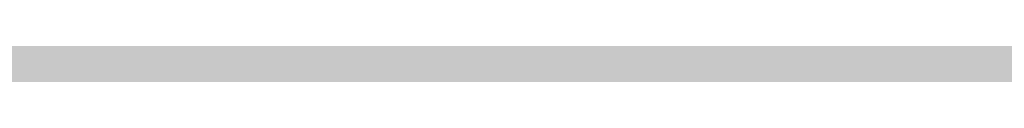
# Model space of a CAD drawing. Units: inches. Extents: x 2091 to 2899, y 967 to 2217.
# Tile 215 of 256: x 2203.2571 to 2203.4104, y 1152.2504 to 1152.2538. Entities that reach past the tile are written whole.
import ezdxf

# ---------------------------------------------------------------- set-up
doc = ezdxf.new("R2010")
doc.units = ezdxf.units.IN
doc.layers.add('A-WALL-PATT', color=141, linetype='Continuous', lineweight=13, true_color=0xadddf7)

msp = doc.modelspace()

# ---------------------------------------------------------------- hatches: boundary and pattern name
at = {"layer": 'A-WALL-PATT'}
h = msp.add_hatch(color=256, dxfattribs=at)
h.dxf.hatch_style = 1
h.paths.add_polyline_path([(2803.1436, 2050.91906), (2203.1436, 2050.91906), (2203.1436, 1090.91906), (2803.1436, 1090.91906)])
h.paths.add_polyline_path([(2635.79885, 1147.54046), (2674.52405, 1147.54046, 0.376086), (2678.52967, 1152.8802), (2678.52967, 1159.55647, 0.333335), (2674.52432, 1163.56185), (2674.52432, 1163.56185), (2674.52432, 1192.93439), (2635.80597, 1192.93439), (2597.08762, 1192.93439), (2597.08762, 1163.56185, 0.333335), (2593.08228, 1159.55647), (2593.08228, 1152.8802, 0.376086), (2597.08789, 1147.54046)], flags=0)
h.paths.add_polyline_path([(2436.01043, 1278.24078, 0.000483), (2435.95264, 1278.21503, -0.001328), (2435.93563, 1278.11169, -0.001711), (2436.11644, 1278.04076, 0.002185)], flags=0)
h.paths.add_polyline_path([(2794.1436, 1143.41906), (2794.1436, 1347.41906), (2543.37017, 1347.41906), (2543.37017, 1351.91906), (2794.1436, 1351.91906), (2794.1436, 1392.71355), (2793.9474, 1392.71355), (2793.9474, 1473.5369), (2794.1436, 1473.5369), (2794.1436, 1531.91906), (2650.1436, 1531.91906), (2650.1436, 1536.41906), (2794.1436, 1536.41906), (2794.1436, 1692.41906), (2609.37561, 1692.41906), (2609.37561, 1644.41906), (2604.87561, 1644.41906), (2604.87561, 1744.91906), (2609.37561, 1744.91906), (2609.37561, 1696.91906), (2794.1436, 1696.91906), (2794.1436, 1780.91906), (2609.6436, 1780.91906), (2493.87561, 1780.91906), (2493.87561, 1785.41906), (2609.6436, 1785.41906), (2794.1436, 1785.41906), (2794.1436, 1847.93882), (2793.95122, 1847.93882), (2793.95122, 1928.76217), (2794.1436, 1928.76217), (2794.1436, 1941.41906), (2614.1436, 1941.41906), (2614.1436, 1821.41906), (2609.6436, 1821.41906), (2609.6436, 1941.41906), (2392.1436, 1941.41906), (2392.1436, 1819.91906), (2387.6436, 1819.91906), (2387.6436, 1941.41906), (2212.1436, 1941.41906), (2212.1436, 1783.91906), (2392.1436, 1783.91906), (2392.1436, 1780.91906), (2212.1436, 1780.91906), (2212.1436, 1629.41906), (2387.6436, 1629.41906), (2387.6436, 1744.91906), (2392.1436, 1744.91906), (2392.1436, 1627.91906), (2317.1436, 1627.91906), (2317.1436, 1551.41906), (2317.1436, 1536.41906), (2459.38359, 1536.41906), (2459.38359, 1602.39648), (2463.88359, 1602.39648), (2463.88359, 1531.91906), (2456.6436, 1531.91906), (2456.6436, 1529.91906), (2452.1436, 1529.91906), (2452.1436, 1531.91906), (2312.6436, 1531.91906), (2312.6436, 1551.41906), (2306.1436, 1551.41906), (2306.1436, 1555.91906), (2308.1436, 1555.91906), (2308.1436, 1551.41906), (2312.6436, 1551.41906), (2312.6436, 1627.91906), (2212.1436, 1627.91906), (2212.1436, 1555.91906), (2270.1436, 1555.91906), (2270.1436, 1551.41906), (2212.1436, 1551.41906), (2212.1436, 1351.91906), (2272.1436, 1351.91906), (2272.1436, 1347.41906), (2212.1436, 1347.41906), (2212.1436, 1275.41906), (2308.1436, 1275.41906), (2308.1436, 1351.91906), (2452.1436, 1351.91906), (2452.1436, 1493.91906), (2456.6436, 1493.91906), (2456.6436, 1347.41906), (2312.6436, 1347.41906), (2312.6436, 1270.91906), (2212.1436, 1270.91906), (2212.1436, 1099.91906), (2281.23752, 1099.91906), (2282.87104, 1110.9138), (2282.00834, 1116.9966), (2278.55774, 1121.4204), (2268.20564, 1128.0562), (2272.08764, 1128.0562), (2273.81294, 1131.927), (2279.42034, 1134.6919), (2285.02784, 1135.2449), (2287.61584, 1137.4568), (2288.04714, 1138.0098), (2289.34114, 1140.7747), (2291.06654, 1139.6687), (2292.36054, 1135.2449), (2295.37984, 1136.9038), (2296.24254, 1135.7979), (2297.10524, 1133.033), (2300.12464, 1138.0098), (2303.14394, 1138.0098), (2304.43794, 1135.7979), (2303.14394, 1133.586), (2306.59464, 1134.6919), (2307.88874, 1133.033), (2310.90804, 1135.2449), (2313.92744, 1134.1389), (2315.62686, 1132.4271), (2308.32004, 1117.5496), (2290.20384, 1109.8079), (2288.90984, 1103.1721), (2289.27231, 1099.91906), (2434.91823, 1099.91906), (2431.59323, 1124.78806), (2429.93023, 1169.55306), (2430.92718, 1240.51969), (2435.65893, 1238.18613), (2437.13523, 1196.55406), (2438.79823, 1143.97306), (2442.67823, 1111.99806), (2446.55823, 1099.91906), (2794.1436, 1099.91906), (2794.1436, 1138.91906), (2548.03245, 1138.91906), (2548.03245, 1143.41906), (2548.03245, 1148.81906), (2546.66846, 1148.03156), (2528.68569, 1179.17862, 0.256256), (2512.03245, 1148.81906), (2512.03245, 1143.41906), (2512.03245, 1138.91906), (2507.53245, 1138.91906), (2507.53245, 1143.41906), (2507.53245, 1148.81906, 0.256256), (2490.8792, 1179.17862), (2472.89644, 1148.03156), (2471.53245, 1148.81906), (2471.53245, 1143.41906), (2467.03245, 1143.41906), (2467.03245, 1269.94579, 0.039061), (2460.90999, 1273.58006), (2467.03245, 1273.58006), (2467.03245, 1286.32536, 0.014511), (2465.21619, 1286.76191), (2467.03245, 1287.05258), (2467.03245, 1323.41906), (2471.53245, 1323.41906), (2471.53245, 1148.81906), (2489.53245, 1179.99597), (2490.89644, 1179.20847), (2490.8792, 1179.17862, -0.256256), (2507.53245, 1148.81906), (2507.53245, 1143.41906), (2512.03245, 1143.41906), (2512.03245, 1148.81906, -0.256256), (2528.68569, 1179.17862), (2528.66846, 1179.20847), (2530.03245, 1179.99597), (2548.03245, 1148.81906), (2548.03245, 1143.41906)], flags=16)
h.paths.add_polyline_path([(2607.76855, 1200.94508), (2607.76855, 1265.03063), (2597.08762, 1281.05201), (2619.78459, 1281.05201), (2627.79528, 1337.12686), (2635.79885, 1337.12686), (2643.81666, 1337.12686), (2651.82736, 1281.05201), (2674.52432, 1281.05201), (2663.8434, 1265.03063), (2663.8434, 1200.94508), (2635.80597, 1200.94508)], flags=0)
edge = h.paths.add_edge_path(flags=0)
edge.add_ellipse((13303.89622, 1272.99872), major_axis=(-10595.31304, 0), ratio=0.84230387009, start_angle=0.628237219, end_angle=0.6465541, ccw=False)
edge.add_ellipse((2711.70045, 1156.85268), major_axis=(2.21977, 0), ratio=0.8423039, start_angle=111.53524, end_angle=180.62824, ccw=False)
edge.add_ellipse((13303.15629, 1272.99872), major_axis=(-10593.02631, 0), ratio=0.84230386954, start_angle=0.528271472, end_angle=0.646554097, ccw=False)
edge.add_line((2710.7646, 1175.3333), (2710.12999, 1175.3333))
edge.add_ellipse((2710.12999, 1176.57978), major_axis=(1.47985, 0), ratio=0.8423039, start_angle=180, end_angle=270, ccw=False)
edge.add_line((2708.65014, 1176.57978), (2708.65014, 1200.78291))
edge.add_ellipse((2710.12999, 1200.78291), major_axis=(1.47985, 0), ratio=0.8423039, start_angle=90, end_angle=180, ccw=False)
edge.add_line((2710.12999, 1202.02939), (2710.46508, 1202.02939))
edge.add_ellipse((13303.15629, 1272.99872), major_axis=(-10593.02631, 0), ratio=0.84230386954, start_angle=-0.090229089, end_angle=0.383866779, ccw=False)
edge.add_ellipse((2710.12999, 1290.92703), major_axis=(-1.47985, 0), ratio=0.8423039, start_angle=0, end_angle=90, ccw=False)
edge.add_line((2708.65014, 1290.92703), (2708.65014, 1315.13017))
edge.add_ellipse((2710.12999, 1315.13017), major_axis=(-1.47985, 0), ratio=0.8423039, start_angle=-90, end_angle=0, ccw=False)
edge.add_line((2710.12999, 1316.37665), (2710.70631, 1316.37665))
edge.add_ellipse((3238.40172, 1296.28957), major_axis=(528.234, 0), ratio=0.84230387, start_angle=176.3495724, end_angle=177.8200497, ccw=False)
edge.add_ellipse((2775.06304, 1071.4507), major_axis=(313.30776, 0), ratio=0.84230387, start_angle=102.1259656, end_angle=103.780529, ccw=False)
edge.add_ellipse((2775.06304, 1078.3057), major_axis=(-305.30289, 0), ratio=0.84230387, start_angle=-79.790461, end_angle=-77.5553727, ccw=False)
edge.add_ellipse((2695.14177, 1541.97538), major_axis=(-250.96022, 0), ratio=0.84230387, start_angle=99.256566, end_angle=102.5549326)
edge.add_line((2741.41033, 1334.21426), (2747.13255, 1337.37848))
edge.add_ellipse((2747.53862, 1336.85748), major_axis=(-0.73992, 0), ratio=0.842304, start_angle=270, end_angle=307.93313, ccw=False)
edge.add_ellipse((2747.53862, 1336.85748), major_axis=(-0.73992, 0), ratio=0.842304, start_angle=232.06687, end_angle=270, ccw=False)
edge.add_line((2747.94469, 1337.37848), (2753.66691, 1334.21426))
edge.add_ellipse((2799.93547, 1541.97538), major_axis=(250.96022, 0), ratio=0.84230387, start_angle=257.4450674, end_angle=260.743434)
edge.add_ellipse((2720.01419, 1078.3057), major_axis=(305.30289, 0), ratio=0.84230387, start_angle=77.5553727, end_angle=79.790461, ccw=False)
edge.add_ellipse((2720.01419, 1071.4507), major_axis=(-313.30776, 0), ratio=0.84230387, start_angle=256.219471, end_angle=257.8740344, ccw=False)
edge.add_ellipse((2256.67551, 1296.28957), major_axis=(-528.234, 0), ratio=0.84230387, start_angle=182.1799503, end_angle=183.6504276, ccw=False)
edge.add_line((2784.37092, 1316.37665), (2784.94725, 1316.37665))
edge.add_ellipse((2784.94725, 1315.13017), major_axis=(1.47985, 0), ratio=0.8423039, start_angle=0, end_angle=90, ccw=False)
edge.add_line((2786.42709, 1315.13017), (2786.42709, 1290.92703))
edge.add_ellipse((2784.94725, 1290.92703), major_axis=(1.47985, 0), ratio=0.8423039, start_angle=270, end_angle=360, ccw=False)
edge.add_ellipse((-7808.07906, 1272.99872), major_axis=(10593.02631, 0), ratio=0.84230386954, start_angle=-0.383866779, end_angle=0.090229089, ccw=False)
edge.add_line((2784.61216, 1202.02939), (2784.94725, 1202.02939))
edge.add_ellipse((2784.94725, 1200.78291), major_axis=(1.47985, 0), ratio=0.8423039, start_angle=0, end_angle=90, ccw=False)
edge.add_line((2786.42709, 1200.78291), (2786.42709, 1176.57978))
edge.add_ellipse((2784.94725, 1176.57978), major_axis=(-1.47985, 0), ratio=0.8423039, start_angle=90, end_angle=180, ccw=False)
edge.add_line((2784.94725, 1175.3333), (2784.31264, 1175.3333))
edge.add_ellipse((-7808.07906, 1272.99872), major_axis=(10593.02631, 0), ratio=0.84230386954, start_angle=-0.618643196, end_angle=-0.528271472, ccw=False)
edge.add_ellipse((2783.37678, 1156.85268), major_axis=(-2.21977, 0), ratio=0.8423039, start_angle=179.37176, end_angle=248.46476, ccw=False)
edge.add_ellipse((-7808.81898, 1272.99872), major_axis=(-10595.31304, 0), ratio=0.84230386576, start_angle=179.353445923, end_angle=179.371762803, ccw=False)
edge.add_ellipse((2780.2973, 1153.50079), major_axis=(-5.24643, 0), ratio=0.8423039, start_angle=90, end_angle=179.35345, ccw=False)
edge.add_line((2780.2973, 1149.08171), (2714.77993, 1149.08171))
edge.add_ellipse((2714.77993, 1153.50079), major_axis=(5.24643, 0), ratio=0.8423039, start_angle=180.64655, end_angle=270, ccw=False)
edge = h.paths.add_edge_path(flags=0)
edge.add_line((2718.18737, 1151.00783), (2718.18737, 1170.47236))
edge.add_ellipse((2721.14706, 1170.47236), major_axis=(-2.95969, 0), ratio=0.8423039, start_angle=-90, end_angle=0, ccw=False)
edge.add_line((2721.14706, 1172.96532), (2773.93017, 1172.96532))
edge.add_ellipse((2773.93017, 1170.47236), major_axis=(-2.95969, 0), ratio=0.8423039, start_angle=180, end_angle=270, ccw=False)
edge.add_line((2776.88987, 1170.47236), (2776.88987, 1151.00783))
edge.add_line((2776.88987, 1151.00783), (2718.18737, 1151.00783))
edge = h.paths.add_edge_path(flags=0)
edge.add_line((2718.18737, 1180.23415), (2718.18737, 1199.05783))
edge.add_ellipse((2747.53862, 1320.39864), major_axis=(147.01792, 0), ratio=0.84230387, start_angle=256.4018653, end_angle=283.5981347)
edge.add_line((2776.88987, 1199.05783), (2776.88987, 1180.23415))
edge.add_ellipse((2747.53862, 1301.57496), major_axis=(147.01792, 0), ratio=0.84230387, start_angle=256.4018653, end_angle=283.5981347, ccw=False)
edge = h.paths.add_edge_path(flags=0)
edge.add_ellipse((13303.15629, 1272.99872), major_axis=(-10591.54646, 0), ratio=0.84230386955, start_angle=0.055594314, end_angle=0.377764194, ccw=False)
edge.add_line((2711.61686, 1262.72171), (2715.66741, 1249.4954))
edge.add_ellipse((6413.89196, 1241.69192), major_axis=(-3698.23616, 0), ratio=0.8423038695, start_angle=-0.12089737, end_angle=0.36407635)
edge.add_line((2715.76104, 1218.19245), (2711.93431, 1203.16736))
edge = h.paths.add_edge_path(flags=0)
edge.add_line((2718.18737, 1251.07457), (2716.00249, 1267.45044))
edge.add_ellipse((2742.15117, 1202.18954), major_axis=(81.77258, 0), ratio=0.84230387, start_angle=94.277421, end_angle=111.8349538, ccw=False)
edge.add_line((2737.00975, 1270.93063), (2758.06748, 1270.93063))
edge.add_ellipse((2752.92606, 1202.18954), major_axis=(81.77258, 0), ratio=0.84230387, start_angle=68.1650462, end_angle=85.722579, ccw=False)
edge.add_line((2779.07475, 1267.45044), (2776.88987, 1251.07457))
edge.add_ellipse((2750.33806, 1187.88536), major_axis=(79.57966, 0), ratio=0.84230387, start_angle=67.2080851, end_angle=85.1299304)
edge.add_line((2756.03466, 1254.74366), (2739.04258, 1254.74366))
edge.add_ellipse((2744.73917, 1187.88536), major_axis=(79.57966, 0), ratio=0.84230387, start_angle=94.8700696, end_angle=112.7919149)
edge = h.paths.add_edge_path(flags=0)
edge.add_line((2783.14293, 1203.16736), (2779.31619, 1218.19245))
edge.add_ellipse((-918.81473, 1241.69192), major_axis=(3698.23616, 0), ratio=0.8423038695, start_angle=-0.36407635, end_angle=0.12089737)
edge.add_line((2779.40983, 1249.4954), (2783.46037, 1262.72171))
edge.add_ellipse((-7808.07906, 1272.99872), major_axis=(-10591.54646, 0), ratio=0.84230386954, start_angle=179.622235806, end_angle=179.944405687, ccw=False)
edge = h.paths.add_edge_path(flags=0)
edge.add_ellipse((2734.20089, 1286.69044), major_axis=(-0.35661, 6.34008), ratio=0.6038336, start_angle=89.002014, end_angle=253.657408, ccw=False)
edge.add_line((2730.369, 1286.54181), (2730.369, 1301.35198))
edge.add_line((2730.369, 1301.35198), (2735.91331, 1305.2148))
edge.add_ellipse((2736.38492, 1304.73456), major_axis=(0.73992, 0), ratio=0.842304, start_angle=90, end_angle=134.48021, ccw=False)
edge.add_line((2736.38492, 1305.3578), (2738.03278, 1305.3578))
edge.add_line((2738.03278, 1305.3578), (2738.03278, 1307.70793))
edge.add_ellipse((2794.20164, 1307.70793), major_axis=(56.16886, 0), ratio=0.84230387, start_angle=150.56143, end_angle=180, ccw=False)
edge.add_ellipse((2700.87559, 1307.70793), major_axis=(-56.16886, 0), ratio=0.84230387, start_angle=180, end_angle=209.43857, ccw=False)
edge.add_line((2757.04445, 1307.70793), (2757.04445, 1305.3578))
edge.add_line((2757.04445, 1305.3578), (2758.69232, 1305.3578))
edge.add_ellipse((2758.69232, 1304.73456), major_axis=(-0.73992, 0), ratio=0.842304, start_angle=225.51979, end_angle=270, ccw=False)
edge.add_line((2759.16392, 1305.2148), (2764.70823, 1301.35198))
edge.add_line((2764.70823, 1301.35198), (2764.70823, 1286.54181))
edge.add_ellipse((2760.87634, 1286.69044), major_axis=(0.35661, 6.34008), ratio=0.6038336, start_angle=106.342592, end_angle=270.997986, ccw=False)
edge.add_line((2757.04445, 1285.79709), (2757.04445, 1307.70793))
edge.add_ellipse((2700.87559, 1307.70793), major_axis=(-56.16886, 0), ratio=0.84230387, start_angle=180, end_angle=209.43857)
edge.add_ellipse((2794.20164, 1307.70793), major_axis=(56.16886, 0), ratio=0.84230387, start_angle=150.56143, end_angle=180)
edge.add_line((2738.03278, 1307.70793), (2738.03278, 1285.79709))
h.paths.add_polyline_path([(2417.81227, 1104.4497), (2413.49227, 1102.5297), (2410.61227, 1103.9697), (2409.17227, 1106.3697), (2407.25227, 1107.3297), (2406.29227, 1109.7297), (2405.33227, 1114.0497), (2405.33227, 1117.8897), (2406.29227, 1120.1297), (2407.25227, 1119.8097), (2408.84832, 1118.32766), (2410.17395, 1119.42417), (2410.21127, 1120.4057), (2411.04073, 1121.41905), (2410.69927, 1119.8587), (2410.17395, 1119.42417), (2410.08845, 1117.17611), (2411.13284, 1116.20632), (2413.97227, 1119.3297), (2416.85227, 1120.7697), (2416.86972, 1120.79878), (2417.03507, 1119.40512), (2417.89621, 1118.14338), (2418.29227, 1118.3697), (2419.54445, 1120.03927), (2419.36092, 1118.38749), (2419.03211, 1119.35615), (2418.39894, 1118.51193), (2419.25227, 1114.5297), (2418.79409, 1107.19879)], flags=0)
h.paths.add_polyline_path([(2508.87017, 1347.41906), (2508.37017, 1347.41906), (2508.37017, 1351.91906), (2508.87017, 1351.91906)], flags=0)
h.paths.add_polyline_path([(2473.37017, 1347.41906), (2472.37017, 1347.41906), (2467.87017, 1347.41906), (2467.87017, 1455.41906), (2472.37017, 1455.41906), (2472.37017, 1352.41906), (2473.37017, 1352.41906)], flags=0)
h.paths.add_polyline_path([(2352.10624, 1217.4462), (2349.22624, 1218.8862), (2347.78624, 1221.2862), (2345.86624, 1222.2462), (2344.90624, 1224.6462), (2343.94624, 1228.9662), (2343.94624, 1232.8062), (2344.90624, 1235.0462), (2345.86624, 1234.7262), (2347.46229, 1233.24415), (2348.78792, 1234.34066), (2348.82524, 1235.3222), (2349.6547, 1236.33555), (2349.31324, 1234.7752), (2348.78792, 1234.34066), (2348.70242, 1232.0926), (2349.74681, 1231.12282), (2352.58624, 1234.2462), (2355.46624, 1235.6862), (2355.48369, 1235.71528), (2355.64904, 1234.32161), (2356.51018, 1233.05988), (2356.90624, 1233.2862), (2358.15842, 1234.95576), (2357.97489, 1233.30398), (2357.64608, 1234.27264), (2357.01291, 1233.42842), (2357.86624, 1229.4462), (2357.40806, 1222.11529), (2356.42624, 1219.3662)], flags=0)
h.paths.add_polyline_path([(2348.2968, 1112.22442), (2347.0138, 1112.31042), (2345.5298, 1114.12742), (2345.7318, 1115.85842), (2346.8118, 1116.98242), (2346.8118, 1114.64642), (2345.8668, 1114.21442), (2346.8798, 1114.30042)], flags=0)
h.paths.add_polyline_path([(2347.0138, 1110.92642), (2346.2718, 1110.49342), (2346.6098, 1111.18642)], flags=0)
h.paths.add_polyline_path([(2345.8668, 1118.19442), (2345.5298, 1117.32942), (2343.7078, 1118.02142), (2344.3828, 1118.62642)], flags=0)
h.paths.add_polyline_path([(2346.6768, 1109.28242), (2346.0698, 1108.07142), (2345.8668, 1110.06142)], flags=0)
h.paths.add_polyline_path([(2345.0568, 1119.75142), (2343.6398, 1119.75142), (2343.9778, 1121.13542)], flags=0)
h.paths.add_polyline_path([(2345.2598, 1116.55042), (2345.1248, 1115.85842), (2344.9218, 1115.68542), (2344.7198, 1116.37742)], flags=0)
h.paths.add_polyline_path([(2345.6648, 1112.31042), (2345.4618, 1111.53242), (2344.0448, 1111.96442), (2344.6518, 1112.57042)], flags=0)
h.paths.add_polyline_path([(2345.1918, 1113.34942), (2344.4498, 1113.86842), (2344.7198, 1114.38742)], flags=0)
h.paths.add_polyline_path([(2344.6518, 1116.80942), (2344.1798, 1115.68542), (2344.6518, 1115.33942), (2343.9098, 1114.90642), (2343.0328, 1115.94442), (2343.6398, 1116.46342)], flags=0)
h.paths.add_polyline_path([(2345.8668, 1106.68642), (2344.9898, 1105.56242), (2344.5168, 1106.60042)], flags=0)
h.paths.add_polyline_path([(2344.8548, 1110.06142), (2344.5168, 1109.28242), (2344.1128, 1109.71542)], flags=0)
h.paths.add_polyline_path([(2344.0448, 1113.52242), (2343.4378, 1113.08942), (2342.7628, 1113.95442)], flags=0)
h.paths.add_polyline_path([(2344.3148, 1111.01242), (2342.9648, 1110.32042), (2342.9648, 1111.09942)], flags=0)
h.paths.add_polyline_path([(2345.1248, 1104.69742), (2344.5848, 1103.74542), (2344.4498, 1104.26442)], flags=0)
h.paths.add_polyline_path([(2342.8298, 1121.22242), (2341.7498, 1120.53042), (2340.5358, 1121.04942), (2340.1308, 1121.82842), (2340.6708, 1122.95242), (2341.1428, 1121.82842), (2341.6148, 1122.00142)], flags=0)
h.paths.add_polyline_path([(2342.9648, 1119.75142), (2343.0328, 1118.45342), (2342.0878, 1118.02142), (2342.0198, 1119.49142)], flags=0)
h.paths.add_polyline_path([(2342.6948, 1116.89642), (2341.9528, 1116.63642), (2342.0198, 1117.32942)], flags=0)
h.paths.add_polyline_path([(2343.0328, 1112.22442), (2342.0198, 1111.79142), (2341.5478, 1112.22442), (2342.3578, 1113.34942)], flags=0)
h.paths.add_polyline_path([(2343.7748, 1104.43742), (2342.6278, 1102.88042), (2342.6948, 1104.61042), (2343.4378, 1105.12942)], flags=0)
h.paths.add_polyline_path([(2342.0198, 1115.07942), (2340.8058, 1115.51242), (2340.9408, 1116.37742)], flags=0)
h.paths.add_polyline_path([(2341.4808, 1120.09742), (2341.4808, 1119.40542), (2341.0758, 1119.57842), (2341.1428, 1120.09742)], flags=0)
h.paths.add_polyline_path([(2341.8178, 1114.47342), (2340.9408, 1113.08942), (2340.8058, 1114.56042)], flags=0)
h.paths.add_polyline_path([(2341.1428, 1118.54042), (2340.9408, 1116.98242), (2339.0508, 1117.67542), (2339.0508, 1118.62642)], flags=0)
h.paths.add_polyline_path([(2342.6948, 1101.66842), (2341.9528, 1101.84142), (2342.5598, 1102.36142)], flags=0)
h.paths.add_polyline_path([(2340.3328, 1119.66542), (2338.4438, 1119.57842), (2337.9038, 1120.35742), (2339.6578, 1120.61642)], flags=0)
h.paths.add_polyline_path([(2340.3328, 1115.33942), (2340.0628, 1113.69542), (2339.3878, 1115.33942)], flags=0)
h.paths.add_polyline_path([(2341.8178, 1103.83142), (2341.5478, 1102.88042), (2341.1428, 1103.65842)], flags=0)
h.paths.add_polyline_path([(2339.0508, 1122.86642), (2337.2958, 1121.82842), (2337.0938, 1123.12542), (2337.7688, 1123.81842)], flags=0)
h.paths.add_polyline_path([(2339.1178, 1121.74142), (2338.8478, 1121.22242), (2338.1738, 1121.04942), (2338.3758, 1121.56842)], flags=0)
h.paths.add_polyline_path([(2339.1858, 1119.31942), (2338.6458, 1118.71342), (2338.2408, 1118.10742), (2338.2408, 1118.88642)], flags=0)
h.paths.add_polyline_path([(2341.1428, 1101.92842), (2340.6028, 1101.23642), (2340.0628, 1101.84142), (2340.6028, 1102.36142)], flags=0)
h.paths.add_polyline_path([(2337.6338, 1117.76142), (2336.6208, 1118.28042), (2337.2958, 1118.97242)], flags=0)
h.paths.add_polyline_path([(2336.8238, 1119.57842), (2334.7988, 1118.97242), (2335.2038, 1120.35742), (2336.5538, 1120.87642)], flags=0)
h.paths.add_polyline_path([(2339.1178, 1100.45742), (2337.3638, 1100.54342), (2336.7558, 1101.23642)], flags=0)
h.paths.add_polyline_path([(2336.3508, 1122.43342), (2336.0138, 1121.91442), (2334.9338, 1122.43342), (2334.5288, 1123.47142), (2335.7438, 1122.77942)], flags=0)
h.paths.add_polyline_path([(2334.7318, 1120.87642), (2334.2588, 1120.35742), (2334.0568, 1120.78942), (2334.5968, 1121.30842)], flags=0)
h.paths.add_polyline_path([(2334.4618, 1122.17442), (2332.5718, 1121.30842), (2331.3568, 1122.17442), (2332.0998, 1122.86642)], flags=0)
h.paths.add_polyline_path([(2334.2588, 1118.54042), (2333.3818, 1118.45342), (2333.6518, 1119.31942)], flags=0)
h.paths.add_polyline_path([(2335.5418, 1102.27442), (2334.1918, 1102.62042), (2335.2718, 1103.31242)], flags=0)
h.paths.add_polyline_path([(2332.7068, 1119.66542), (2331.6948, 1120.44342), (2332.5048, 1120.78942)], flags=0)
h.paths.add_polyline_path([(2334.7318, 1101.14942), (2333.5168, 1101.58242), (2333.9888, 1101.75542)], flags=0)
h.paths.add_polyline_path([(2332.6398, 1116.63642), (2331.0868, 1116.29042), (2331.9648, 1118.19442)], flags=0)
h.paths.add_polyline_path([(2330.7498, 1121.56842), (2330.2768, 1120.27042), (2328.5228, 1119.31942), (2328.9948, 1121.04942)], flags=0)
h.paths.add_polyline_path([(2330.7498, 1118.62642), (2330.0078, 1117.50242), (2329.8728, 1118.02142)], flags=0)
h.paths.add_polyline_path([(2332.0998, 1102.36142), (2330.5468, 1102.01442), (2331.6948, 1102.96642)], flags=0)
h.paths.add_polyline_path([(2329.5348, 1113.60842), (2329.0628, 1112.31042), (2328.5898, 1113.34942)], flags=0)
h.paths.add_polyline_path([(2328.3878, 1117.84842), (2327.5098, 1116.55042), (2327.1728, 1117.76142)], flags=0)
h.paths.add_polyline_path([(2329.7378, 1106.51342), (2329.5348, 1105.30242), (2328.2528, 1106.08142)], flags=0)
h.paths.add_polyline_path([(2328.6578, 1114.38742), (2328.0498, 1114.12742), (2328.3198, 1114.90642)], flags=0)
h.paths.add_polyline_path([(2328.3198, 1112.22442), (2327.1058, 1112.13742), (2326.7008, 1112.65642)], flags=0)
h.paths.add_polyline_path([(2326.9028, 1115.25242), (2326.7008, 1114.12742), (2325.2158, 1113.60842), (2326.0928, 1115.33942)], flags=0)
h.paths.add_polyline_path([(2326.6328, 1108.33042), (2326.0928, 1107.37942), (2325.8908, 1108.50342), (2326.4978, 1109.10942)], flags=0)
h.paths.add_polyline_path([(2615.1436, 1531.91906), (2609.6436, 1531.91906), (2609.6436, 1620.41906), (2614.1436, 1620.41906), (2614.1436, 1536.41906), (2615.1436, 1536.41906)], flags=0)
h.paths.add_polyline_path([(2545.1436, 1563.41906), (2464.1436, 1563.41906), (2464.1436, 1632.41906), (2509.1436, 1632.41906), (2509.1436, 1627.91906), (2509.1436, 1603.91906), (2468.6436, 1603.91906), (2468.6436, 1567.91906), (2540.6436, 1567.91906), (2540.6436, 1591.91906), (2545.1436, 1591.91906)], flags=0)
h.paths.add_polyline_path([(2388.96905, 1549.98573), (2357.43418, 1549.98573), (2357.43418, 1623.36078), (2399.36278, 1623.36078), (2435.68947, 1623.36078), (2435.59255, 1602.55927), (2435.59255, 1602.39648), (2388.96905, 1602.39648)], flags=0)
h.paths.add_polyline_path([(2388.88063, 1555.80915), (2374.90443, 1555.80915), (2374.90443, 1600.57156), (2374.90443, 1615.45765), (2406.35088, 1615.45765), (2406.35088, 1618.93943), (2412.17429, 1615.45765), (2406.35088, 1611.97586), (2406.35088, 1615.45765), (2388.88063, 1615.45765)], flags=0)
h.paths.add_polyline_path([(2568.87561, 1644.41906), (2453.37561, 1644.41906), (2453.37561, 1785.41906), (2457.87561, 1785.41906), (2457.87561, 1648.91906), (2568.87561, 1648.91906)], flags=0)
h.paths.add_polyline_path([(2212.1436, 1945.91906), (2212.1436, 2041.91906), (2794.1436, 2041.91906), (2794.1436, 1945.91906)], flags=16)
h.paths.add_polyline_path([(2271.08273, 1964.31724), (2776.85297, 1964.31724), (2776.85297, 2037.16962), (2271.08273, 2037.16962)], flags=8)
h.paths.add_polyline_path([(2380.64929, 1536.82414), (2461.04081, 1536.82414), (2461.04081, 1554.65259), (2380.64929, 1554.65259)], flags=8)
h.paths.add_polyline_path([(2240.75571, 1609.72545), (2309.18583, 1609.72545), (2309.18583, 1617.6982), (2240.75571, 1617.6982)], flags=8)
h.paths.add_polyline_path([(2212.67726, 1313.5041), (2282.59152, 1313.5041), (2282.59152, 1322.74524), (2212.67726, 1322.74524)], flags=8)
h.paths.add_polyline_path([(2457.11198, 1114.77857), (2558.48158, 1114.77857), (2558.48158, 1142.21968), (2457.11198, 1142.21968)], flags=8)
h.paths.add_polyline_path([(2473.44234, 1273.01007), (2604.64123, 1273.01007), (2604.64123, 1318.34693), (2473.44234, 1318.34693)], flags=8)
h.paths.add_polyline_path([(2638.8763, 1626.97743), (2684.25037, 1627.97674), (2684.03848, 1637.59749), (2638.66442, 1636.59819)], flags=8)
h.paths.add_polyline_path([(2537.59055, 1453.79345), (2628.38955, 1453.79345), (2628.38955, 1475.34481), (2537.59055, 1475.34481)], flags=8)
h.paths.add_polyline_path([(2504.13764, 1714.6324), (2554.64719, 1714.6324), (2554.64719, 1730.23771), (2504.13764, 1730.23771)], flags=8)
h.paths.add_polyline_path([(2487.50118, 1575.65187), (2535.09712, 1575.65187), (2535.09712, 1598.37765), (2487.50118, 1598.37765)], flags=8)
h.paths.add_polyline_path([(2709.0994, 1735.71028), (2740.0166, 1735.71028), (2740.0166, 1749.93764), (2709.0994, 1749.93764)], flags=8)
h.paths.add_polyline_path([(2442.43842, 1792.17166), (2564.72884, 1792.17166), (2564.72884, 1842.00016), (2442.43842, 1842.00016)], flags=8)
h.paths.add_polyline_path([(2655.8158, 1809.64408), (2789.52014, 1806.6938), (2790.08498, 1832.29164), (2656.38064, 1835.24192)], flags=8)
h.paths.add_polyline_path([(2234.8427, 1797.72014), (2368.59285, 1794.76885), (2369.16072, 1820.50413), (2235.41056, 1823.45542)], flags=8)
h.paths.add_polyline_path([(2245.13847, 1644.00633), (2398.42773, 1640.6239), (2398.99484, 1666.32482), (2245.70557, 1669.70725)], flags=8)
h.paths.add_polyline_path([(2306.14285, 1431.16852), (2413.76831, 1428.79369), (2414.33315, 1454.39153), (2306.70768, 1456.76636)], flags=8)
h.paths.add_polyline_path([(2306.83458, 1458.23314), (2393.38048, 1456.32345), (2393.93281, 1481.35436), (2307.38691, 1483.26405)], flags=8)

doc.saveas('drawing.dxf')
